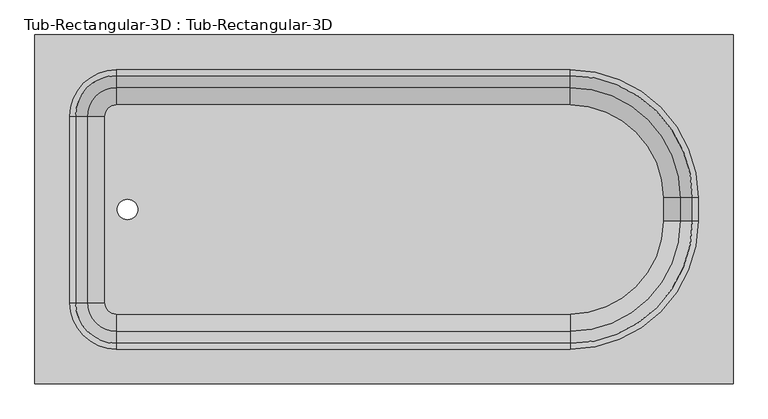
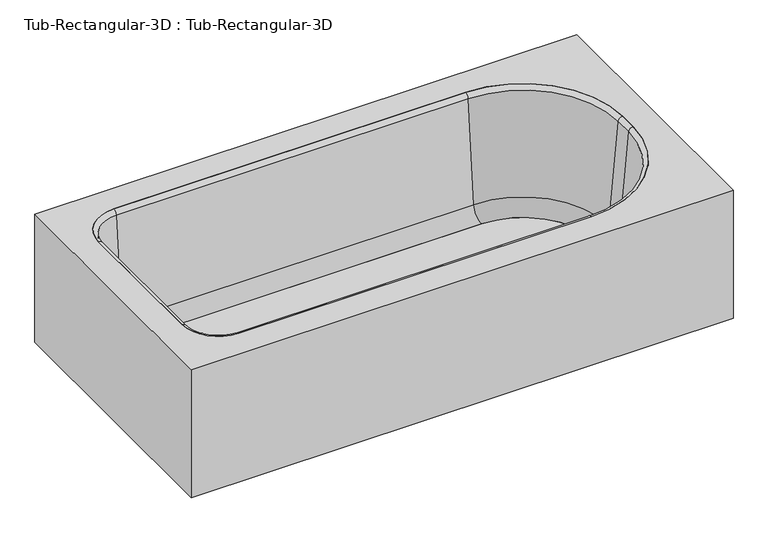
"""IFC4 building model written with IfcOpenShell, lengths in millimetres: flow terminal geometry, Tub-Rectangular-3D : Tub-Rectangular-3D."""

from ifc_helpers import new_model, si_unit, point, frame, frame_2d, origin, place, context, project, spatial, polyline, circle_curve, ellipse_curve, trimmed, segment, composite_curve, outline, extrude, source, transform, mapped, element, save
from ifc_brep_helpers import plane_surface, cylinder_surface, revolved_surface, advanced_brep


def tub_rectangular_3d_tub_rectangular_3d_ca47631e(model_context):
    return source(origin(), model_context, "Body", "SolidModel", [
        advanced_brep(
        [(413.3970313, 863.6, 381.0), (-1110.6029687, 863.6, 381.0), (-1110.6029687, 101.6, 381.0), (413.3970313, 101.6, 381.0), (-932.8029687, 787.4, 381.0), (57.7970313, 787.4, 381.0), (337.1970313, 508.0, 381.0), (337.1970313, 457.2, 381.0), (57.7970313, 177.8, 381.0), (-932.8029687, 177.8, 381.0), (-1034.4029687, 279.4, 381.0), (-1034.4029687, 685.8, 381.0), (394.3470313, 844.55, 361.95), (394.3470313, 120.65, 361.95), (-1091.5529687, 120.65, 361.95), (-1091.5529687, 844.55, 361.95), (-932.8029687, 787.4, 361.95), (-1034.4029687, 685.8, 361.95), (-1034.4029687, 279.4, 361.95), (-932.8029687, 177.8, 361.95), (57.7970313, 177.8, 361.95), (337.1970313, 457.2, 361.95), (337.1970313, 508.0, 361.95), (57.7970313, 787.4, 361.95), (413.3970313, 863.6, 0.0), (-1110.6029687, 863.6, 0.0), (-1110.6029687, 101.6, 0.0), (413.3970313, 101.6, 0.0), (394.3470313, 844.55, 0.0), (-1091.5529687, 844.55, 0.0), (-1091.5529687, 120.65, 0.0), (394.3470313, 120.65, 0.0)],
        [
            (0, 1),
            (1, 2),
            (2, 3),
            (3, 0),
            (4, 5),
            (5, 6, circle_curve(frame((57.7970313, 508.0, 381.0), z_axis=(0.0, 0.0, -1.0), x_axis=(0.0, 1.0, 0.0)), 279.4)),
            (6, 7),
            (7, 8, circle_curve(frame((57.7970313, 457.2, 381.0), z_axis=(0.0, 0.0, -1.0), x_axis=(0.0, 1.0, 0.0)), 279.4)),
            (8, 9),
            (9, 10, circle_curve(frame((-932.8029687, 279.4, 381.0), z_axis=(0.0, 0.0, -1.0), x_axis=(0.0, 1.0, 0.0)), 101.6)),
            (10, 11),
            (11, 4, circle_curve(frame((-932.8029687, 685.8, 381.0), z_axis=(0.0, 0.0, -1.0), x_axis=(0.0, 1.0, 0.0)), 101.6)),
            (12, 13),
            (13, 14),
            (14, 15),
            (15, 12),
            (16, 17, circle_curve(frame((-932.8029687, 685.8, 361.95), z_axis=(0.0, 0.0, 1.0), x_axis=(0.0, 1.0, 0.0)), 101.6)),
            (17, 18),
            (18, 19, circle_curve(frame((-932.8029687, 279.4, 361.95), z_axis=(0.0, 0.0, 1.0), x_axis=(0.0, 1.0, 0.0)), 101.6)),
            (19, 20),
            (20, 21, circle_curve(frame((57.7970313, 457.2, 361.95), z_axis=(0.0, 0.0, 1.0), x_axis=(0.0, 1.0, 0.0)), 279.4)),
            (21, 22),
            (22, 23, circle_curve(frame((57.7970313, 508.0, 361.95), z_axis=(0.0, 0.0, 1.0), x_axis=(0.0, 1.0, 0.0)), 279.4)),
            (23, 16),
            (0, 24),
            (24, 25),
            (25, 1),
            (25, 26),
            (26, 2),
            (26, 27),
            (27, 3),
            (27, 24),
            (4, 16),
            (23, 5),
            (22, 6),
            (21, 7),
            (20, 8),
            (19, 9),
            (18, 10),
            (17, 11),
            (28, 29),
            (29, 30),
            (30, 31),
            (31, 28),
            (31, 13),
            (12, 28),
            (30, 14),
            (29, 15),
        ],
        [
            plane_surface(frame((-1110.6029687, 863.6, 381.0), z_axis=(0.0, 0.0, 1.0), x_axis=(-1.0, 0.0, 0.0))),
            plane_surface(frame((-1110.6029687, 863.6, 361.95), z_axis=(0.0, 0.0, -1.0), x_axis=(1.0, 0.0, 0.0))),
            plane_surface(frame((413.3970313, 863.6, 381.0), z_axis=(0.0, 1.0, 0.0), x_axis=(0.0, 0.0, -1.0))),
            plane_surface(frame((-1110.6029687, 863.6, 381.0), z_axis=(-1.0, 0.0, 0.0), x_axis=(0.0, 0.0, -1.0))),
            plane_surface(frame((-1110.6029687, 101.6, 381.0), z_axis=(0.0, -1.0, 0.0), x_axis=(0.0, 0.0, -1.0))),
            plane_surface(frame((413.3970313, 101.6, 381.0), z_axis=(1.0, 0.0, 0.0), x_axis=(0.0, 0.0, -1.0))),
            plane_surface(frame((-932.8029687, 787.4, 381.0), z_axis=(0.0, -1.0, 0.0), x_axis=(0.0, 0.0, -1.0))),
            revolved_surface(polyline([(57.7970313, 787.4, 361.95), (57.7970313, 787.4, 381.0)]), (57.7970313, 508.0, 381.0), (0.0, 0.0, -1.0)),
            plane_surface(frame((337.1970313, 508.0, 381.0), z_axis=(-1.0, 0.0, 0.0), x_axis=(0.0, 0.0, -1.0))),
            revolved_surface(polyline([(57.7970313, 736.5999999999999, 361.95), (57.7970313, 736.5999999999999, 381.0)]), (57.7970313, 457.2, 381.0), (0.0, 0.0, -1.0)),
            plane_surface(frame((57.7970313, 177.8, 381.0), z_axis=(0.0, 1.0, 0.0), x_axis=(0.0, 0.0, -1.0))),
            revolved_surface(polyline([(-932.8029687, 381.0, 361.95), (-932.8029687, 381.0, 381.0)]), (-932.8029687, 279.4, 381.0), (0.0, 0.0, -1.0)),
            plane_surface(frame((-1034.4029687, 279.4, 381.0), z_axis=(1.0, 0.0, 0.0), x_axis=(0.0, 0.0, -1.0))),
            revolved_surface(polyline([(-932.8029687, 787.4, 361.95), (-932.8029687, 787.4, 381.0)]), (-932.8029687, 685.8, 381.0), (0.0, 0.0, -1.0)),
            plane_surface(frame((-1110.6029687, 863.6, 0.0), z_axis=(0.0, 0.0, -1.0), x_axis=(1.0, 0.0, 0.0))),
            plane_surface(frame((394.3470313, 844.55, 361.95), z_axis=(-1.0, 0.0, 0.0), x_axis=(0.0, 0.0, -1.0))),
            plane_surface(frame((394.3470313, 120.65, 361.95), z_axis=(0.0, 1.0, 0.0), x_axis=(0.0, 0.0, -1.0))),
            plane_surface(frame((-1091.5529687, 120.65, 361.95), z_axis=(1.0, 0.0, 0.0), x_axis=(0.0, 0.0, -1.0))),
            plane_surface(frame((-1091.5529687, 844.55, 361.95), z_axis=(0.0, -1.0, 0.0), x_axis=(0.0, 0.0, -1.0))),
        ],
        [
            (0, [[1, 2, 3, 4], [5, 6, 7, 8, 9, 10, 11, 12]]),
            (1, [[13, 14, 15, 16], [17, 18, 19, 20, 21, 22, 23, 24]]),
            (2, [[-1, 25, 26, 27]]),
            (3, [[-2, -27, 28, 29]]),
            (4, [[-3, -29, 30, 31]]),
            (5, [[-25, -4, -31, 32]]),
            (6, [[-5, 33, -24, 34]]),
            (7, [[-6, -34, -23, 35]]),
            (8, [[-7, -35, -22, 36]]),
            (9, [[-8, -36, -21, 37]]),
            (10, [[-9, -37, -20, 38]]),
            (11, [[-10, -38, -19, 39]]),
            (12, [[-11, -39, -18, 40]]),
            (13, [[-12, -40, -17, -33]]),
            (14, [[-32, -30, -28, -26], [41, 42, 43, 44]]),
            (15, [[-44, 45, -13, 46]]),
            (16, [[-43, 47, -14, -45]]),
            (17, [[-42, 48, -15, -47]]),
            (18, [[-41, -46, -16, -48]]),
        ],
    ),
        extrude(outline(composite_curve([segment(trimmed(circle_curve(frame_2d((57.7970313, 508.0)), 202.7964741), [point((57.7970313, 710.7964741))], [point((260.5935054, 508.0))], False, "CARTESIAN"), True, "CONTINUOUS"), segment(polyline([(260.5935054, 508.0), (260.5935054, 457.2)]), True, "CONTINUOUS"), segment(trimmed(circle_curve(frame_2d((57.7970313, 457.2)), 202.7964741), [point((260.5935054, 457.2))], [point((57.7970313, 254.4035259))], False, "CARTESIAN"), True, "CONTINUOUS"), segment(polyline([(57.7970313, 254.4035259), (-932.8029687, 254.4035259)]), True, "CONTINUOUS"), segment(trimmed(circle_curve(frame_2d((-932.8029687, 279.4)), 24.9964741), [point((-932.8029687, 254.4035259))], [point((-957.7994428, 279.4))], False, "CARTESIAN"), True, "CONTINUOUS"), segment(polyline([(-957.7994428, 279.4), (-957.7994428, 685.8)]), True, "CONTINUOUS"), segment(trimmed(circle_curve(frame_2d((-932.8029687, 685.8)), 24.9964741), [point((-957.7994428, 685.8))], [point((-932.8029687, 710.7964741))], False, "CARTESIAN"), True, "CONTINUOUS"), segment(polyline([(-932.8029687, 710.7964741), (57.7970313, 710.7964741)]), True, "CONTINUOUS")], self_intersect=False), holes=[composite_curve([segment(trimmed(circle_curve(frame_2d((-908.510206, 482.6)), 22.225), [point((-908.510206, 504.825))], [point((-908.510206, 460.375))], True, "CARTESIAN"), True, "CONTINUOUS"), segment(trimmed(circle_curve(frame_2d((-908.510206, 482.6)), 22.225), [point((-908.510206, 460.375))], [point((-908.510206, 504.825))], True, "CARTESIAN"), True, "CONTINUOUS")], self_intersect=False)]), frame((0.0, 0.0, 16.863573), z_axis=(0.0, 0.0, 1.0), x_axis=(1.0, 0.0, 0.0)), (0.0, 0.0, 1.0), 19.05),
        advanced_brep(
        [(-995.7544608, 685.8, 70.6929392), (-932.8029687, 748.7514921, 70.6929392), (-932.8029687, 774.9220035, 369.8232535), (-1021.9249722, 685.8, 369.8232535), (-957.7994428, 685.8, 35.913573), (-932.8029687, 710.7964741, 35.913573), (-957.7994428, 685.8, 16.863573), (-932.8029687, 710.7964741, 16.863573), (-1034.4029687, 685.8, 16.863573), (-932.8029687, 787.4, 16.863573), (-1034.4029687, 685.8, 381.0), (-932.8029687, 787.4, 381.0), (-1021.9249722, 279.4, 369.8232535), (-995.7544608, 279.4, 70.6929392), (-957.7994428, 279.4, 35.913573), (-957.7994428, 279.4, 16.863573), (-1034.4029687, 279.4, 16.863573), (-1034.4029687, 279.4, 381.0), (-932.8029687, 216.4485079, 70.6929392), (-932.8029687, 190.2779965, 369.8232535), (-932.8029687, 254.4035259, 35.913573), (-932.8029687, 254.4035259, 16.863573), (-932.8029687, 177.8, 16.863573), (-932.8029687, 177.8, 381.0), (57.7970313, 190.2779965, 369.8232535), (57.7970313, 216.4485079, 70.6929392), (57.7970313, 254.4035259, 35.913573), (57.7970313, 254.4035259, 16.863573), (57.7970313, 177.8, 16.863573), (57.7970313, 177.8, 381.0), (298.5485234, 457.2, 70.6929392), (324.7190348, 457.2, 369.8232535), (260.5935054, 457.2, 35.913573), (260.5935054, 457.2, 16.863573), (337.1970313, 457.2, 16.863573), (337.1970313, 457.2, 381.0), (324.7190348, 508.0, 369.8232535), (298.5485234, 508.0, 70.6929392), (260.5935054, 508.0, 35.913573), (260.5935054, 508.0, 16.863573), (337.1970313, 508.0, 16.863573), (337.1970313, 508.0, 381.0), (57.7970313, 748.7514921, 70.6929392), (57.7970313, 774.9220035, 369.8232535), (57.7970313, 710.7964741, 35.913573), (57.7970313, 710.7964741, 16.863573), (57.7970313, 787.4, 16.863573), (57.7970313, 787.4, 381.0)],
        [
            (0, 1, circle_curve(frame((-932.8029687, 685.8, 70.6929392), z_axis=(0.0, 0.0, -1.0), x_axis=(0.0, 1.0, 0.0)), 62.9514921)),
            (1, 2),
            (2, 3, circle_curve(frame((-932.8029687, 685.8, 369.8232535), z_axis=(0.0, 0.0, 1.0), x_axis=(0.0, 1.0, 0.0)), 89.1220035)),
            (3, 0),
            (4, 5, circle_curve(frame((-932.8029687, 685.8, 35.913573), z_axis=(0.0, 0.0, -1.0), x_axis=(0.0, 1.0, 0.0)), 24.9964741)),
            (5, 1, circle_curve(frame((-932.8029687, 710.7964741, 74.013573), z_axis=(1.0, 0.0, 0.0), x_axis=(0.0, -1.0, 0.0)), 38.1)),
            (0, 4, circle_curve(frame((-957.7994428, 685.8, 74.013573), z_axis=(0.0, -1.0, 0.0), x_axis=(1.0, 0.0, 0.0)), 38.1)),
            (6, 7, circle_curve(frame((-932.8029687, 685.8, 16.863573), z_axis=(0.0, 0.0, -1.0), x_axis=(0.0, 1.0, 0.0)), 24.9964741)),
            (7, 5),
            (4, 6),
            (8, 9, circle_curve(frame((-932.8029687, 685.8, 16.863573), z_axis=(0.0, 0.0, -1.0), x_axis=(0.0, 1.0, 0.0)), 101.6)),
            (9, 7),
            (6, 8),
            (10, 11, circle_curve(frame((-932.8029687, 685.8, 381.0), z_axis=(0.0, 0.0, -1.0), x_axis=(0.0, 1.0, 0.0)), 101.6)),
            (11, 9),
            (8, 10),
            (2, 11, circle_curve(frame((-932.8029687, 787.4, 368.4462547), z_axis=(-1.0, 0.0, 0.0), x_axis=(0.0, -1.0, 0.0)), 12.5537453)),
            (10, 3, circle_curve(frame((-1034.4029687, 685.8, 368.4462547), z_axis=(0.0, 1.0, 0.0), x_axis=(1.0, 0.0, 0.0)), 12.5537453)),
            (3, 12),
            (12, 13),
            (13, 0),
            (13, 14, circle_curve(frame((-957.7994428, 279.4, 74.013573), z_axis=(0.0, -1.0, 0.0), x_axis=(1.0, 0.0, 0.0)), 38.1)),
            (14, 4),
            (14, 15),
            (15, 6),
            (15, 16),
            (16, 8),
            (16, 17),
            (17, 10),
            (17, 12, circle_curve(frame((-1034.4029687, 279.4, 368.4462547), z_axis=(0.0, 1.0, 0.0), x_axis=(1.0, 0.0, 0.0)), 12.5537453)),
            (18, 13, circle_curve(frame((-932.8029687, 279.4, 70.6929392), z_axis=(0.0, 0.0, -1.0), x_axis=(-1.0, 0.0, 0.0)), 62.9514921)),
            (12, 19, circle_curve(frame((-932.8029687, 279.4, 369.8232535), z_axis=(0.0, 0.0, 1.0), x_axis=(-1.0, 0.0, 0.0)), 89.1220035)),
            (19, 18),
            (20, 14, circle_curve(frame((-932.8029687, 279.4, 35.913573), z_axis=(0.0, 0.0, -1.0), x_axis=(-1.0, 0.0, 0.0)), 24.9964741)),
            (18, 20, circle_curve(frame((-932.8029687, 254.4035259, 74.013573), z_axis=(1.0, 0.0, 0.0), x_axis=(0.0, 1.0, 0.0)), 38.1)),
            (21, 15, circle_curve(frame((-932.8029687, 279.4, 16.863573), z_axis=(0.0, 0.0, -1.0), x_axis=(-1.0, 0.0, 0.0)), 24.9964741)),
            (20, 21),
            (22, 16, circle_curve(frame((-932.8029687, 279.4, 16.863573), z_axis=(0.0, 0.0, -1.0), x_axis=(-1.0, 0.0, 0.0)), 101.6)),
            (21, 22),
            (23, 17, circle_curve(frame((-932.8029687, 279.4, 381.0), z_axis=(0.0, 0.0, -1.0), x_axis=(-1.0, 0.0, 0.0)), 101.6)),
            (22, 23),
            (23, 19, circle_curve(frame((-932.8029687, 177.8, 368.4462547), z_axis=(-1.0, 0.0, 0.0), x_axis=(0.0, 1.0, 0.0)), 12.5537453)),
            (19, 24),
            (24, 25),
            (25, 18),
            (25, 26, circle_curve(frame((57.7970313, 254.4035259, 74.013573), z_axis=(1.0, 0.0, 0.0), x_axis=(0.0, 1.0, 0.0)), 38.1)),
            (26, 20),
            (26, 27),
            (27, 21),
            (27, 28),
            (28, 22),
            (28, 29),
            (29, 23),
            (29, 24, circle_curve(frame((57.7970313, 177.8, 368.4462547), z_axis=(-1.0, 0.0, 0.0), x_axis=(0.0, 1.0, 0.0)), 12.5537453)),
            (30, 25, circle_curve(frame((57.7970313, 457.2, 70.6929392), z_axis=(0.0, 0.0, -1.0), x_axis=(0.0, -1.0, 0.0)), 240.7514921)),
            (24, 31, circle_curve(frame((57.7970313, 457.2, 369.8232535), z_axis=(0.0, 0.0, 1.0), x_axis=(0.0, -1.0, 0.0)), 266.9220035)),
            (31, 30),
            (32, 26, circle_curve(frame((57.7970313, 457.2, 35.913573), z_axis=(0.0, 0.0, -1.0), x_axis=(0.0, -1.0, 0.0)), 202.7964741)),
            (30, 32, circle_curve(frame((260.5935054, 457.2, 74.013573), z_axis=(0.0, 1.0, 0.0), x_axis=(-1.0, 0.0, 0.0)), 38.1)),
            (33, 27, circle_curve(frame((57.7970313, 457.2, 16.863573), z_axis=(0.0, 0.0, -1.0), x_axis=(0.0, -1.0, 0.0)), 202.7964741)),
            (32, 33),
            (34, 28, circle_curve(frame((57.7970313, 457.2, 16.863573), z_axis=(0.0, 0.0, -1.0), x_axis=(0.0, -1.0, 0.0)), 279.4)),
            (33, 34),
            (35, 29, circle_curve(frame((57.7970313, 457.2, 381.0), z_axis=(0.0, 0.0, -1.0), x_axis=(0.0, -1.0, 0.0)), 279.4)),
            (34, 35),
            (35, 31, circle_curve(frame((337.1970313, 457.2, 368.4462547), z_axis=(0.0, -1.0, 0.0), x_axis=(-1.0, 0.0, 0.0)), 12.5537453)),
            (31, 36),
            (36, 37),
            (37, 30),
            (37, 38, circle_curve(frame((260.5935054, 508.0, 74.013573), z_axis=(0.0, 1.0, 0.0), x_axis=(-1.0, 0.0, 0.0)), 38.1)),
            (38, 32),
            (38, 39),
            (39, 33),
            (39, 40),
            (40, 34),
            (40, 41),
            (41, 35),
            (41, 36, circle_curve(frame((337.1970313, 508.0, 368.4462547), z_axis=(0.0, -1.0, 0.0), x_axis=(-1.0, 0.0, 0.0)), 12.5537453)),
            (42, 37, circle_curve(frame((57.7970313, 508.0, 70.6929392), z_axis=(0.0, 0.0, -1.0), x_axis=(1.0, 0.0, 0.0)), 240.7514921)),
            (36, 43, circle_curve(frame((57.7970313, 508.0, 369.8232535), z_axis=(0.0, 0.0, 1.0), x_axis=(1.0, 0.0, 0.0)), 266.9220035)),
            (43, 42),
            (44, 38, circle_curve(frame((57.7970313, 508.0, 35.913573), z_axis=(0.0, 0.0, -1.0), x_axis=(1.0, 0.0, 0.0)), 202.7964741)),
            (42, 44, circle_curve(frame((57.7970313, 710.7964741, 74.013573), z_axis=(-1.0, 0.0, 0.0), x_axis=(0.0, -1.0, 0.0)), 38.1)),
            (45, 39, circle_curve(frame((57.7970313, 508.0, 16.863573), z_axis=(0.0, 0.0, -1.0), x_axis=(1.0, 0.0, 0.0)), 202.7964741)),
            (44, 45),
            (46, 40, circle_curve(frame((57.7970313, 508.0, 16.863573), z_axis=(0.0, 0.0, -1.0), x_axis=(1.0, 0.0, 0.0)), 279.4)),
            (45, 46),
            (47, 41, circle_curve(frame((57.7970313, 508.0, 381.0), z_axis=(0.0, 0.0, -1.0), x_axis=(1.0, 0.0, 0.0)), 279.4)),
            (46, 47),
            (47, 43, circle_curve(frame((57.7970313, 787.4, 368.4462547), z_axis=(1.0, 0.0, 0.0), x_axis=(0.0, -1.0, 0.0)), 12.5537453)),
            (43, 2),
            (1, 42),
            (5, 44),
            (7, 45),
            (9, 46),
            (11, 47),
        ],
        [
            revolved_surface(polyline([(-932.8029687, 774.9220035, 369.8232535), (-932.8029687, 748.7514921, 70.6929392)]), (-932.8029687, 685.8, 381.0), (0.0, 0.0, 1.0)),
            revolved_surface(trimmed(ellipse_curve(frame((-932.8029687, 710.7964741, 74.013573), z_axis=(-1.0, 0.0, 0.0), x_axis=(0.0, -1.0, 0.0)), 38.1, 38.1), [point((-932.8029687, 748.7514921, 70.6929392))], [point((-932.8029687, 710.7964741, 35.913573))], True, "CARTESIAN"), (-932.8029687, 685.8, 381.0), (0.0, 0.0, 1.0)),
            revolved_surface(polyline([(-932.8029687, 710.7964741, 35.913572999999985), (-932.8029687, 710.7964741, 16.863572999999974)]), (-932.8029687, 685.8, 381.0), (0.0, 0.0, 1.0)),
            plane_surface(frame((-932.8029687, 685.8, 16.863573), z_axis=(0.0, 0.0, -1.0), x_axis=(0.0, 1.0, 0.0))),
            cylinder_surface(frame((-932.8029687, 685.8, 381.0), z_axis=(0.0, 0.0, 1.0), x_axis=(0.0, 1.0, 0.0)), 101.6),
            revolved_surface(trimmed(ellipse_curve(frame((-932.8029687, 787.4, 368.4462547), z_axis=(1.0, 0.0, 0.0), x_axis=(0.0, -1.0, 0.0)), 12.5537453, 12.5537453), [point((-932.8029687, 787.4, 381.0))], [point((-932.8029687, 774.9220035, 369.8232535))], True, "CARTESIAN"), (-932.8029687, 685.8, 381.0), (0.0, 0.0, 1.0)),
            plane_surface(frame((-1021.9249722, 685.8, 369.8232535), z_axis=(0.9961946980917458, 0.0, 0.08715574274765589), x_axis=(0.0, -1.0, 0.0))),
            revolved_surface(polyline([(-919.6994427999999, 279.4, 74.013573), (-919.6994427999999, 685.8, 74.013573)]), (-957.7994428, 685.8, 74.013573), (0.0, -1.0, 0.0)),
            plane_surface(frame((-957.7994428, 685.8, 35.913573), z_axis=(1.0, 0.0, 0.0), x_axis=(0.0, -1.0, 0.0))),
            plane_surface(frame((-957.7994428, 685.8, 16.863573), z_axis=(0.0, 0.0, -1.0), x_axis=(0.0, -1.0, 0.0))),
            plane_surface(frame((-1034.4029687, 685.8, 16.863573), z_axis=(-1.0, 0.0, 0.0), x_axis=(0.0, -1.0, 0.0))),
            cylinder_surface(frame((-1034.4029687, 685.8, 368.4462547), z_axis=(0.0, 1.0, 0.0), x_axis=(1.0, 0.0, 0.0)), 12.5537453),
            revolved_surface(polyline([(-1021.9249722, 279.4, 369.8232535), (-995.7544608, 279.4, 70.6929392)]), (-932.8029687, 279.4, 381.0), (0.0, 0.0, 1.0)),
            revolved_surface(trimmed(ellipse_curve(frame((-957.7994428, 279.4, 74.013573), z_axis=(0.0, -1.0, 0.0), x_axis=(1.0, 0.0, 0.0)), 38.1, 38.1), [point((-995.7544608, 279.4, 70.6929392))], [point((-957.7994428, 279.4, 35.913573))], True, "CARTESIAN"), (-932.8029687, 279.4, 381.0), (0.0, 0.0, 1.0)),
            revolved_surface(polyline([(-957.7994428, 279.4, 35.913572999999985), (-957.7994428, 279.4, 16.863572999999974)]), (-932.8029687, 279.4, 381.0), (0.0, 0.0, 1.0)),
            plane_surface(frame((-932.8029687, 279.4, 16.863573), z_axis=(0.0, 0.0, -1.0), x_axis=(-1.0, 0.0, 0.0))),
            cylinder_surface(frame((-932.8029687, 279.4, 381.0), z_axis=(0.0, 0.0, 1.0), x_axis=(-1.0, 0.0, 0.0)), 101.6),
            revolved_surface(trimmed(ellipse_curve(frame((-1034.4029687, 279.4, 368.4462547), z_axis=(0.0, 1.0, 0.0), x_axis=(1.0, 0.0, 0.0)), 12.5537453, 12.5537453), [point((-1034.4029687, 279.4, 381.0))], [point((-1021.9249722, 279.4, 369.8232535))], True, "CARTESIAN"), (-932.8029687, 279.4, 381.0), (0.0, 0.0, 1.0)),
            plane_surface(frame((-932.8029687, 190.2779965, 369.8232535), z_axis=(0.0, 0.9961946980917461, 0.08715574274765266), x_axis=(1.0, 0.0, 0.0))),
            revolved_surface(polyline([(57.79703129999996, 292.5035259, 74.013573), (-932.8029687, 292.5035259, 74.013573)]), (-932.8029687, 254.4035259, 74.013573), (1.0, 0.0, 0.0)),
            plane_surface(frame((-932.8029687, 254.4035259, 35.913573), z_axis=(0.0, 1.0, 0.0), x_axis=(1.0, 0.0, 0.0))),
            plane_surface(frame((-932.8029687, 254.4035259, 16.863573), z_axis=(0.0, 0.0, -1.0), x_axis=(1.0, 0.0, 0.0))),
            plane_surface(frame((-932.8029687, 177.8, 16.863573), z_axis=(0.0, -1.0, 0.0), x_axis=(1.0, 0.0, 0.0))),
            cylinder_surface(frame((-932.8029687, 177.8, 368.4462547), z_axis=(-1.0, 0.0, 0.0), x_axis=(0.0, 1.0, 0.0)), 12.5537453),
            revolved_surface(polyline([(57.7970313, 190.2779965, 369.8232535), (57.7970313, 216.4485079, 70.6929392)]), (57.7970313, 457.2, 381.0), (0.0, 0.0, 1.0)),
            revolved_surface(trimmed(ellipse_curve(frame((57.7970313, 254.4035259, 74.013573), z_axis=(1.0, 0.0, 0.0), x_axis=(0.0, 1.0, 0.0)), 38.1, 38.1), [point((57.7970313, 216.4485079, 70.6929392))], [point((57.7970313, 254.4035259, 35.913573))], True, "CARTESIAN"), (57.7970313, 457.2, 381.0), (0.0, 0.0, 1.0)),
            revolved_surface(polyline([(57.7970313, 254.40352589999998, 35.913572999999985), (57.7970313, 254.40352589999998, 16.863572999999974)]), (57.7970313, 457.2, 381.0), (0.0, 0.0, 1.0)),
            plane_surface(frame((57.7970313, 457.2, 16.863573), z_axis=(0.0, 0.0, -1.0), x_axis=(0.0, -1.0, 0.0))),
            cylinder_surface(frame((57.7970313, 457.2, 381.0), z_axis=(0.0, 0.0, 1.0), x_axis=(0.0, -1.0, 0.0)), 279.4),
            revolved_surface(trimmed(ellipse_curve(frame((57.7970313, 177.8, 368.4462547), z_axis=(-1.0, 0.0, 0.0), x_axis=(0.0, 1.0, 0.0)), 12.5537453, 12.5537453), [point((57.7970313, 177.8, 381.0))], [point((57.7970313, 190.2779965, 369.8232535))], True, "CARTESIAN"), (57.7970313, 457.2, 381.0), (0.0, 0.0, 1.0)),
            plane_surface(frame((324.7190348, 457.2, 369.8232535), z_axis=(-0.9961946980917464, 0.0, 0.08715574274764942), x_axis=(0.0, 1.0, 0.0))),
            revolved_surface(polyline([(222.49350540000003, 508.0, 74.013573), (222.49350540000003, 457.2, 74.013573)]), (260.5935054, 457.2, 74.013573), (0.0, 1.0, 0.0)),
            plane_surface(frame((260.5935054, 457.2, 35.913573), z_axis=(-1.0, 0.0, 0.0), x_axis=(0.0, 1.0, 0.0))),
            plane_surface(frame((260.5935054, 457.2, 16.863573), z_axis=(0.0, 0.0, -1.0), x_axis=(0.0, 1.0, 0.0))),
            plane_surface(frame((337.1970313, 457.2, 16.863573), z_axis=(1.0, 0.0, 0.0), x_axis=(0.0, 1.0, 0.0))),
            cylinder_surface(frame((337.1970313, 457.2, 368.4462547), z_axis=(0.0, -1.0, 0.0), x_axis=(-1.0, 0.0, 0.0)), 12.5537453),
            revolved_surface(polyline([(324.7190348, 508.0, 369.8232535), (298.5485234, 508.0, 70.6929392)]), (57.7970313, 508.0, 381.0), (0.0, 0.0, 1.0)),
            revolved_surface(trimmed(ellipse_curve(frame((260.5935054, 508.0, 74.013573), z_axis=(0.0, 1.0, 0.0), x_axis=(-1.0, 0.0, 0.0)), 38.1, 38.1), [point((298.5485234, 508.0, 70.6929392))], [point((260.5935054, 508.0, 35.913573))], True, "CARTESIAN"), (57.7970313, 508.0, 381.0), (0.0, 0.0, 1.0)),
            revolved_surface(polyline([(260.5935054, 508.0, 35.913572999999985), (260.5935054, 508.0, 16.863572999999974)]), (57.7970313, 508.0, 381.0), (0.0, 0.0, 1.0)),
            plane_surface(frame((57.7970313, 508.0, 16.863573), z_axis=(0.0, 0.0, -1.0), x_axis=(1.0, 0.0, 0.0))),
            cylinder_surface(frame((57.7970313, 508.0, 381.0), z_axis=(0.0, 0.0, 1.0), x_axis=(1.0, 0.0, 0.0)), 279.4),
            revolved_surface(trimmed(ellipse_curve(frame((337.1970313, 508.0, 368.4462547), z_axis=(0.0, -1.0, 0.0), x_axis=(-1.0, 0.0, 0.0)), 12.5537453, 12.5537453), [point((337.1970313, 508.0, 381.0))], [point((324.7190348, 508.0, 369.8232535))], True, "CARTESIAN"), (57.7970313, 508.0, 381.0), (0.0, 0.0, 1.0)),
            plane_surface(frame((57.7970313, 774.9220035, 369.8232535), z_axis=(0.0, -0.9961946980917461, 0.08715574274765266), x_axis=(-1.0, 0.0, 0.0))),
            revolved_surface(polyline([(-932.8029687, 672.6964740999999, 74.013573), (57.7970313, 672.6964740999999, 74.013573)]), (57.7970313, 710.7964741, 74.013573), (-1.0, 0.0, 0.0)),
            plane_surface(frame((57.7970313, 710.7964741, 35.913573), z_axis=(0.0, -1.0, 0.0), x_axis=(-1.0, 0.0, 0.0))),
            plane_surface(frame((57.7970313, 710.7964741, 16.863573), z_axis=(0.0, 0.0, -1.0), x_axis=(-1.0, 0.0, 0.0))),
            plane_surface(frame((57.7970313, 787.4, 16.863573), z_axis=(0.0, 1.0, 0.0), x_axis=(-1.0, 0.0, 0.0))),
            cylinder_surface(frame((57.7970313, 787.4, 368.4462547), z_axis=(1.0, 0.0, 0.0), x_axis=(0.0, -1.0, 0.0)), 12.5537453),
        ],
        [
            (0, [[1, 2, 3, 4]]),
            (1, [[5, 6, -1, 7]]),
            (2, [[8, 9, -5, 10]]),
            (3, [[11, 12, -8, 13]]),
            (4, [[14, 15, -11, 16]]),
            (5, [[-3, 17, -14, 18]]),
            (6, [[-4, 19, 20, 21]]),
            (7, [[-7, -21, 22, 23]]),
            (8, [[-10, -23, 24, 25]]),
            (9, [[-13, -25, 26, 27]]),
            (10, [[-16, -27, 28, 29]]),
            (11, [[-18, -29, 30, -19]]),
            (12, [[31, -20, 32, 33]]),
            (13, [[34, -22, -31, 35]]),
            (14, [[36, -24, -34, 37]]),
            (15, [[38, -26, -36, 39]]),
            (16, [[40, -28, -38, 41]]),
            (17, [[-32, -30, -40, 42]]),
            (18, [[-33, 43, 44, 45]]),
            (19, [[-35, -45, 46, 47]]),
            (20, [[-37, -47, 48, 49]]),
            (21, [[-39, -49, 50, 51]]),
            (22, [[-41, -51, 52, 53]]),
            (23, [[-42, -53, 54, -43]]),
            (24, [[55, -44, 56, 57]]),
            (25, [[58, -46, -55, 59]]),
            (26, [[60, -48, -58, 61]]),
            (27, [[62, -50, -60, 63]]),
            (28, [[64, -52, -62, 65]]),
            (29, [[-56, -54, -64, 66]]),
            (30, [[-57, 67, 68, 69]]),
            (31, [[-59, -69, 70, 71]]),
            (32, [[-61, -71, 72, 73]]),
            (33, [[-63, -73, 74, 75]]),
            (34, [[-65, -75, 76, 77]]),
            (35, [[-66, -77, 78, -67]]),
            (36, [[79, -68, 80, 81]]),
            (37, [[82, -70, -79, 83]]),
            (38, [[84, -72, -82, 85]]),
            (39, [[86, -74, -84, 87]]),
            (40, [[88, -76, -86, 89]]),
            (41, [[-80, -78, -88, 90]]),
            (42, [[-81, 91, -2, 92]]),
            (43, [[-83, -92, -6, 93]]),
            (44, [[-85, -93, -9, 94]]),
            (45, [[-87, -94, -12, 95]]),
            (46, [[-89, -95, -15, 96]]),
            (47, [[-90, -96, -17, -91]]),
        ],
    ),
    ])


if __name__ == "__main__":
    model = new_model("IFC4")
    model_context = context("Model", 3, world=origin())
    ifc_project = project(units=[si_unit("LENGTHUNIT", "METRE", prefix="MILLI")], contexts=[model_context])
    site = spatial("IfcSite", under=ifc_project)
    building = spatial("IfcBuilding", under=site)
    placement = place(None, origin())
    tub_rectangular_3d_tub_rectangular_3d_shape = tub_rectangular_3d_tub_rectangular_3d_ca47631e(model_context)
    element("IfcFlowTerminal", 1, ObjectType="Tub-Rectangular-3D : Tub-Rectangular-3D", at=placement, inside=building, context=model_context, shape_type="MappedRepresentation", body=[
        mapped(tub_rectangular_3d_tub_rectangular_3d_shape, transform((0.0, 0.0, 0.0), x_axis=(1.0, 0.0, 0.0), y_axis=(0.0, 1.0, 0.0), z_axis=(0.0, 0.0, 1.0))),
    ])
    save(model, "model.ifc")

# Revit data of these elements
# Type "Tub-Rectangular-3D : Tub-Rectangular-3D"
#   Assembly Code = "D2010500"
#   Depth = 2' - 6"
#   Height = 1' - 3"
#   Width = 5' - 0"
#   Tub Material = Porcelain, Ivory
#   Default Elevation = 0
# Element 1 (IfcFlowTerminal, "Tub-Rectangular-3D : Tub-Rectangular-3D")
#   Materials on its faces: "Porcelain, Ivory"
# Materials
#   "Porcelain, Ivory": class "Ceramic", colour RGB 247 247 239, transparency 0, Description = "Porcelain, ivory", Cost = 0
